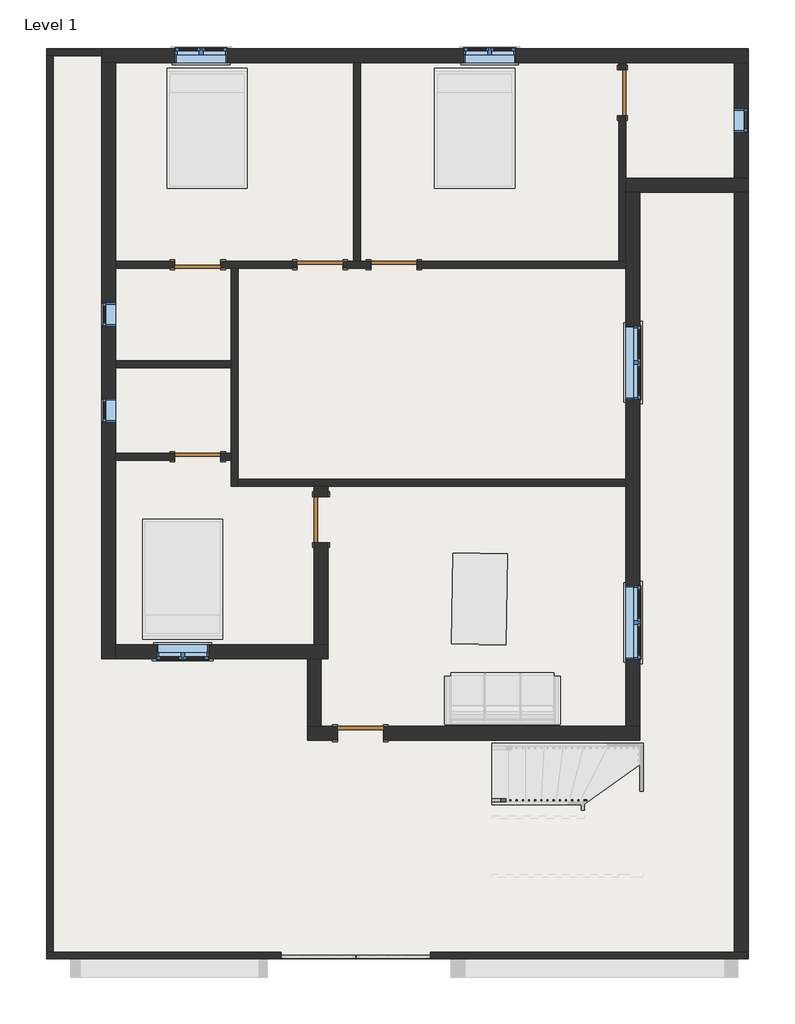
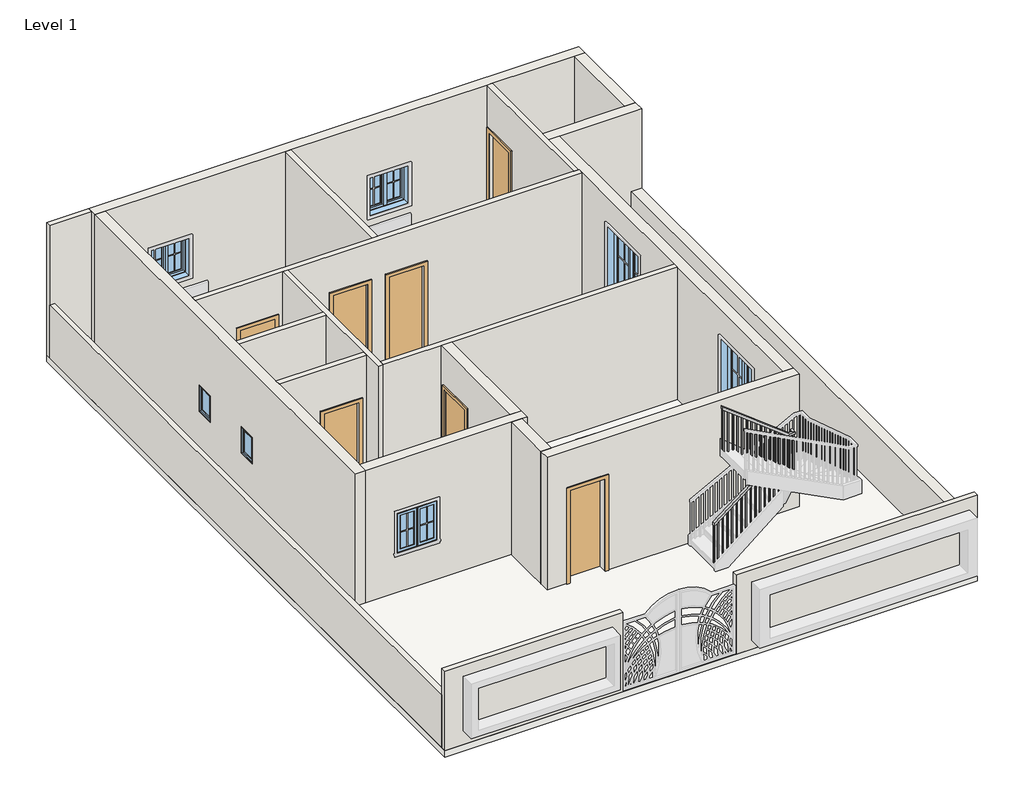
# One storey, part 1 of 2: 21 walls, 8 windows, 7 doors, 1 railing, 1 slab.
"""IFC4 building model written with IfcOpenShell, lengths in millimetres."""

from ifc_helpers import new_model, si_unit, frame, origin, origin_with_axes, place, context, project, spatial, polyline, outline, extrude, faceted_brep, transform, mapped, element, save
from components import door_f2b275c1, door_d8f5dbb5, door_214872d5, door_78caadf7, door_bb98abfd, window_aa618e30, window_339605e1, window_8377141f

model = new_model("IFC4")

# Units and contexts
model_context = context("Model", 3, world=origin())
ifc_project = project(units=[si_unit("LENGTHUNIT", "METRE", prefix="MILLI")], contexts=[model_context])

# Site, building, storey
site = spatial("IfcSite", under=ifc_project)
building = spatial("IfcBuilding", under=site)
storey = spatial("IfcBuildingStorey", under=building, Name="Level 1", Elevation=0.0)

# Doors
placement = place(None, origin())
door_shape = door_f2b275c1(model_context)
element("IfcDoor", 1, ObjectType="Single-Flush : 30\" x 80\"", at=placement, inside=storey, context=model_context, shape_type="MappedRepresentation", body=[
    mapped(door_shape, transform((2459.5084916, 7319.9935985, 0.0), x_axis=(0.0, 1.0, 0.0), y_axis=(-1.0, 0.0, 0.0), z_axis=(0.0, 0.0, 1.0))),
])
element("IfcDoor", 2, ObjectType="Single-Flush : 30\" x 80\"", at=placement, inside=storey, context=model_context, shape_type="MappedRepresentation", body=[
    mapped(door_shape, transform((-4550.8915084, 4481.5435985, 0.0), x_axis=(1.0, 0.0, 0.0), y_axis=(0.0, 1.0, 0.0), z_axis=(0.0, 0.0, 1.0))),
])
door_2_shape = door_d8f5dbb5(model_context)
element("IfcDoor", 3, ObjectType="Single-Flush : 30\" x 80\"", at=placement, inside=storey, context=model_context, shape_type="MappedRepresentation", body=[
    mapped(door_2_shape, transform((-4550.8915084, 1319.2435985, 0.0), x_axis=(1.0, 0.0, 0.0), y_axis=(0.0, 1.0, 0.0), z_axis=(0.0, 0.0, 1.0))),
])
door_3_shape = door_214872d5(model_context)
element("IfcDoor", 4, ObjectType="Single-Flush : 30\" x 84\"", at=placement, inside=storey, context=model_context, shape_type="MappedRepresentation", body=[
    mapped(door_3_shape, transform((-2531.5915084, 4481.5435985, 0.0), x_axis=(1.0, 0.0, 0.0), y_axis=(0.0, 1.0, 0.0), z_axis=(0.0, 0.0, 1.0))),
])
door_4_shape = door_78caadf7(model_context)
element("IfcDoor", 5, ObjectType="Single-Flush : 30\" x 84\"", at=placement, inside=storey, context=model_context, shape_type="MappedRepresentation", body=[
    mapped(door_4_shape, transform((-1312.3915084, 4481.5435985, 0.0), x_axis=(-1.0, 0.0, 0.0), y_axis=(0.0, -1.0, 0.0), z_axis=(0.0, 0.0, 1.0))),
])
door_5_shape = door_bb98abfd(model_context)
element("IfcDoor", 6, ObjectType="Single-Flush : 30\" x 84\"", at=placement, inside=storey, context=model_context, shape_type="MappedRepresentation", body=[
    mapped(door_5_shape, transform((-2512.5415084, 277.8435985, 0.0), x_axis=(0.0, 1.0, 0.0), y_axis=(-1.0, 0.0, 0.0), z_axis=(0.0, 0.0, 1.0))),
])
element("IfcDoor", 7, ObjectType="Single-Flush : 30\" x 84\"", at=placement, inside=storey, context=model_context, shape_type="MappedRepresentation", body=[
    mapped(door_5_shape, transform((-1864.8415084, -3246.4064015, 0.0), x_axis=(1.0, 0.0, 0.0), y_axis=(0.0, 1.0, 0.0), z_axis=(0.0, 0.0, 1.0))),
])

# Railing
element("IfcRailing", 8, ObjectType="Handrail - Rectangular", at=placement, inside=storey, context=model_context, shape_type="SolidModel", body=[
    faceted_brep([(306.9570026, -4325.9064015, 1083.7333333), (306.9570026, -4325.9064015, 1019.4000346), (306.9570026, -4376.7064015, 1019.4000346), (306.9570026, -4376.7064015, 1083.7333333), (1758.4886944, -4325.9064015, 2211.6191036), (1809.2886944, -4325.9064015, 2186.7590024), (1809.2886944, -4376.7064015, 2186.7590024), (1758.4886944, -4376.7064015, 2211.6191036), (1758.4886944, -4325.9064015, 2414.6281882), (1809.2886944, -4325.9064015, 2363.8281882), (1809.2886944, -4376.7064015, 2363.8281882), (1758.4886944, -4376.7064015, 2414.6281882), (1885.4886944, -4325.9064015, 2414.6281882), (1885.4886944, -4325.9064015, 2363.8281882), (1834.6886944, -4376.7064015, 2363.8281882), (1834.6886944, -4376.7064015, 2414.6281882), (1885.4886944, -4452.9064015, 2414.6281882), (1885.4886944, -4482.0277354, 2363.8281882), (1834.6886944, -4482.0277354, 2363.8281882), (1834.6886944, -4452.9064015, 2414.6281882), (1885.4886944, -4579.9064015, 2631.5051451), (1885.4886944, -4630.7064015, 2617.7256424), (1834.6886944, -4630.7064015, 2617.7256424), (1834.6886944, -4579.9064015, 2631.5051451), (1885.4886944, -4579.9064015, 2834.5142297), (1885.4886944, -4630.7064015, 2783.7142297), (1834.6886944, -4630.7064015, 2783.7142297), (1834.6886944, -4579.9064015, 2834.5142297), (1885.4886944, -4706.9064015, 2834.5142297), (1885.4886944, -4706.9064015, 2783.7142297), (1834.6886944, -4656.1064015, 2783.7142297), (1834.6886944, -4656.1064015, 2834.5142297), (1758.4886944, -4706.9064015, 2834.5142297), (1741.0720265, -4706.9064015, 2783.7142297), (1741.0720265, -4656.1064015, 2783.7142297), (1758.4886944, -4656.1064015, 2834.5142297), (306.9570026, -4706.9064015, 3962.4), (306.9570026, -4656.1064015, 3962.4), (306.9570026, -4656.1064015, 3898.0667013), (306.9570026, -4706.9064015, 3898.0667013)], [[[0, 1, 2, 3]], [[1, 0, 4, 5]], [[2, 1, 5, 6]], [[3, 2, 6, 7]], [[0, 3, 7, 4]], [[5, 4, 8, 9]], [[6, 5, 9, 10]], [[7, 6, 10, 11]], [[4, 7, 11, 8]], [[9, 8, 12, 13]], [[10, 9, 13, 14]], [[11, 10, 14, 15]], [[8, 11, 15, 12]], [[13, 12, 16, 17]], [[14, 13, 17, 18]], [[15, 14, 18, 19]], [[12, 15, 19, 16]], [[17, 16, 20, 21]], [[18, 17, 21, 22]], [[19, 18, 22, 23]], [[16, 19, 23, 20]], [[21, 20, 24, 25]], [[22, 21, 25, 26]], [[23, 22, 26, 27]], [[20, 23, 27, 24]], [[25, 24, 28, 29]], [[26, 25, 29, 30]], [[27, 26, 30, 31]], [[24, 27, 31, 28]], [[29, 28, 32, 33]], [[30, 29, 33, 34]], [[31, 30, 34, 35]], [[28, 31, 35, 32]], [[36, 37, 38, 39]], [[33, 32, 36, 39]], [[34, 33, 39, 38]], [[35, 34, 38, 37]], [[32, 35, 37, 36]]]),
    extrude(outline(polyline([(3868.0292361, 345.6136944), (3882.8316852, 326.5636944), (2878.6666667, 326.5636944), (2878.6666667, 345.6136944), (3868.0292361, 345.6136944)])), frame((0.0, -4691.0314015, 0.0), z_axis=(0.0, 1.0, 0.0), x_axis=(0.0, 0.0, 1.0)), (0.0, 0.0, 1.0), 19.05),
    extrude(outline(polyline([(3789.0828411, 447.2136944), (3803.8852902, 428.1636944), (2878.6666667, 428.1636944), (2878.6666667, 447.2136944), (3789.0828411, 447.2136944)])), frame((0.0, -4691.0314015, 0.0), z_axis=(0.0, 1.0, 0.0), x_axis=(0.0, 0.0, 1.0)), (0.0, 0.0, 1.0), 19.05),
    extrude(outline(polyline([(3710.1364462, 548.8136944), (3724.9388952, 529.7636944), (2878.6666667, 529.7636944), (2878.6666667, 548.8136944), (3710.1364462, 548.8136944)])), frame((0.0, -4691.0314015, 0.0), z_axis=(0.0, 1.0, 0.0), x_axis=(0.0, 0.0, 1.0)), (0.0, 0.0, 1.0), 19.05),
    extrude(outline(polyline([(3631.1900512, 650.4136944), (3645.9925003, 631.3636944), (2709.3333333, 631.3636944), (2709.3333333, 650.4136944), (3631.1900512, 650.4136944)])), frame((0.0, -4691.0314015, 0.0), z_axis=(0.0, 1.0, 0.0), x_axis=(0.0, 0.0, 1.0)), (0.0, 0.0, 1.0), 19.05),
    extrude(outline(polyline([(3552.2436562, 752.0136944), (3567.0461053, 732.9636944), (2709.3333333, 732.9636944), (2709.3333333, 752.0136944), (3552.2436562, 752.0136944)])), frame((0.0, -4691.0314015, 0.0), z_axis=(0.0, 1.0, 0.0), x_axis=(0.0, 0.0, 1.0)), (0.0, 0.0, 1.0), 19.05),
    extrude(outline(polyline([(3473.2972613, 853.6136944), (3488.0997103, 834.5636944), (2709.3333333, 834.5636944), (2709.3333333, 853.6136944), (3473.2972613, 853.6136944)])), frame((0.0, -4691.0314015, 0.0), z_axis=(0.0, 1.0, 0.0), x_axis=(0.0, 0.0, 1.0)), (0.0, 0.0, 1.0), 19.05),
    extrude(outline(polyline([(3394.3508663, 955.2136944), (3409.1533154, 936.1636944), (2540.0, 936.1636944), (2540.0, 955.2136944), (3394.3508663, 955.2136944)])), frame((0.0, -4691.0314015, 0.0), z_axis=(0.0, 1.0, 0.0), x_axis=(0.0, 0.0, 1.0)), (0.0, 0.0, 1.0), 19.05),
    extrude(outline(polyline([(3315.4044713, 1056.8136944), (3330.2069204, 1037.7636944), (2540.0, 1037.7636944), (2540.0, 1056.8136944), (3315.4044713, 1056.8136944)])), frame((0.0, -4691.0314015, 0.0), z_axis=(0.0, 1.0, 0.0), x_axis=(0.0, 0.0, 1.0)), (0.0, 0.0, 1.0), 19.05),
    extrude(outline(polyline([(3236.4580764, 1158.4136944), (3251.2605254, 1139.3636944), (2370.6666667, 1139.3636944), (2370.6666667, 1158.4136944), (3236.4580764, 1158.4136944)])), frame((0.0, -4691.0314015, 0.0), z_axis=(0.0, 1.0, 0.0), x_axis=(0.0, 0.0, 1.0)), (0.0, 0.0, 1.0), 19.05),
    extrude(outline(polyline([(3157.5116814, 1260.0136944), (3172.3141304, 1240.9636944), (2370.6666667, 1240.9636944), (2370.6666667, 1260.0136944), (3157.5116814, 1260.0136944)])), frame((0.0, -4691.0314015, 0.0), z_axis=(0.0, 1.0, 0.0), x_axis=(0.0, 0.0, 1.0)), (0.0, 0.0, 1.0), 19.05),
    extrude(outline(polyline([(3078.5652864, 1361.6136944), (3093.3677355, 1342.5636944), (2370.6666667, 1342.5636944), (2370.6666667, 1361.6136944), (3078.5652864, 1361.6136944)])), frame((0.0, -4691.0314015, 0.0), z_axis=(0.0, 1.0, 0.0), x_axis=(0.0, 0.0, 1.0)), (0.0, 0.0, 1.0), 19.05),
    extrude(outline(polyline([(2999.6188914, 1463.2136944), (3014.4213405, 1444.1636944), (2201.3333333, 1444.1636944), (2201.3333333, 1463.2136944), (2999.6188914, 1463.2136944)])), frame((0.0, -4691.0314015, 0.0), z_axis=(0.0, 1.0, 0.0), x_axis=(0.0, 0.0, 1.0)), (0.0, 0.0, 1.0), 19.05),
    extrude(outline(polyline([(2920.6724965, 1564.8136944), (2935.4749455, 1545.7636944), (2201.3333333, 1545.7636944), (2201.3333333, 1564.8136944), (2920.6724965, 1564.8136944)])), frame((0.0, -4691.0314015, 0.0), z_axis=(0.0, 1.0, 0.0), x_axis=(0.0, 0.0, 1.0)), (0.0, 0.0, 1.0), 19.05),
    extrude(outline(polyline([(2841.7261015, 1666.4136944), (2856.5285506, 1647.3636944), (2032.0, 1647.3636944), (2032.0, 1666.4136944), (2841.7261015, 1666.4136944)])), frame((0.0, -4691.0314015, 0.0), z_axis=(0.0, 1.0, 0.0), x_axis=(0.0, 0.0, 1.0)), (0.0, 0.0, 1.0), 19.05),
    extrude(outline(polyline([(2762.7797065, 1768.0136944), (2777.5821556, 1748.9636944), (2032.0, 1748.9636944), (2032.0, 1768.0136944), (2762.7797065, 1768.0136944)])), frame((0.0, -4691.0314015, 0.0), z_axis=(0.0, 1.0, 0.0), x_axis=(0.0, 0.0, 1.0)), (0.0, 0.0, 1.0), 19.05),
    extrude(outline(polyline([(1850.5636944, -4646.5814015), (1869.6136944, -4646.5814015), (1869.6136944, -4665.6314015), (1850.5636944, -4665.6314015), (1850.5636944, -4646.5814015)])), frame((0.0, 0.0, 1693.3333333), z_axis=(0.0, 0.0, 1.0), x_axis=(1.0, 0.0, 0.0)), (0.0, 0.0, 1.0), 1090.3808964),
    extrude(outline(polyline([(-4564.0314015, 2503.86524), (-4544.9814015, 2471.3336964), (-4544.9814015, 1524.0), (-4564.0314015, 1524.0), (-4564.0314015, 2503.86524)])), frame((1850.5636944, 0.0, 0.0), z_axis=(1.0, 0.0, 0.0), x_axis=(0.0, 1.0, 0.0)), (0.0, 0.0, 1.0), 19.05),
    extrude(outline(polyline([(-4462.4314015, 2330.3636744), (-4443.3814015, 2297.8321309), (-4443.3814015, 1354.6666667), (-4462.4314015, 1354.6666667), (-4462.4314015, 2330.3636744)])), frame((1850.5636944, 0.0, 0.0), z_axis=(1.0, 0.0, 0.0), x_axis=(0.0, 1.0, 0.0)), (0.0, 0.0, 1.0), 19.05),
    extrude(outline(polyline([(1821.4320026, -4360.8314015), (1821.4320026, -4341.7814015), (1840.4820026, -4341.7814015), (1840.4820026, -4360.8314015), (1821.4320026, -4360.8314015)])), frame((0.0, 0.0, 1185.3333333), z_axis=(0.0, 0.0, 1.0), x_axis=(1.0, 0.0, 0.0)), (0.0, 0.0, 1.0), 1178.4948549),
    extrude(outline(polyline([(2132.0507888, 1738.8820026), (2117.2483397, 1719.8320026), (1016.0, 1719.8320026), (1016.0, 1738.8820026), (2132.0507888, 1738.8820026)])), frame((0.0, -4360.8314015, 0.0), z_axis=(0.0, 1.0, 0.0), x_axis=(0.0, 0.0, 1.0)), (0.0, 0.0, 1.0), 19.05),
    extrude(outline(polyline([(2053.1043938, 1637.2820026), (2038.3019447, 1618.2320026), (1016.0, 1618.2320026), (1016.0, 1637.2820026), (2053.1043938, 1637.2820026)])), frame((0.0, -4360.8314015, 0.0), z_axis=(0.0, 1.0, 0.0), x_axis=(0.0, 0.0, 1.0)), (0.0, 0.0, 1.0), 19.05),
    extrude(outline(polyline([(1974.1579988, 1535.6820026), (1959.3555498, 1516.6320026), (846.6666667, 1516.6320026), (846.6666667, 1535.6820026), (1974.1579988, 1535.6820026)])), frame((0.0, -4360.8314015, 0.0), z_axis=(0.0, 1.0, 0.0), x_axis=(0.0, 0.0, 1.0)), (0.0, 0.0, 1.0), 19.05),
    extrude(outline(polyline([(1895.2116039, 1434.0820026), (1880.4091548, 1415.0320026), (846.6666667, 1415.0320026), (846.6666667, 1434.0820026), (1895.2116039, 1434.0820026)])), frame((0.0, -4360.8314015, 0.0), z_axis=(0.0, 1.0, 0.0), x_axis=(0.0, 0.0, 1.0)), (0.0, 0.0, 1.0), 19.05),
    extrude(outline(polyline([(1816.2652089, 1332.4820026), (1801.4627598, 1313.4320026), (677.3333333, 1313.4320026), (677.3333333, 1332.4820026), (1816.2652089, 1332.4820026)])), frame((0.0, -4360.8314015, 0.0), z_axis=(0.0, 1.0, 0.0), x_axis=(0.0, 0.0, 1.0)), (0.0, 0.0, 1.0), 19.05),
    extrude(outline(polyline([(1737.3188139, 1230.8820026), (1722.5163649, 1211.8320026), (677.3333333, 1211.8320026), (677.3333333, 1230.8820026), (1737.3188139, 1230.8820026)])), frame((0.0, -4360.8314015, 0.0), z_axis=(0.0, 1.0, 0.0), x_axis=(0.0, 0.0, 1.0)), (0.0, 0.0, 1.0), 19.05),
    extrude(outline(polyline([(1658.3724189, 1129.2820026), (1643.5699699, 1110.2320026), (508.0, 1110.2320026), (508.0, 1129.2820026), (1658.3724189, 1129.2820026)])), frame((0.0, -4360.8314015, 0.0), z_axis=(0.0, 1.0, 0.0), x_axis=(0.0, 0.0, 1.0)), (0.0, 0.0, 1.0), 19.05),
    extrude(outline(polyline([(1579.426024, 1027.6820026), (1564.6235749, 1008.6320026), (508.0, 1008.6320026), (508.0, 1027.6820026), (1579.426024, 1027.6820026)])), frame((0.0, -4360.8314015, 0.0), z_axis=(0.0, 1.0, 0.0), x_axis=(0.0, 0.0, 1.0)), (0.0, 0.0, 1.0), 19.05),
    extrude(outline(polyline([(1500.479629, 926.0820026), (1485.6771799, 907.0320026), (508.0, 907.0320026), (508.0, 926.0820026), (1500.479629, 926.0820026)])), frame((0.0, -4360.8314015, 0.0), z_axis=(0.0, 1.0, 0.0), x_axis=(0.0, 0.0, 1.0)), (0.0, 0.0, 1.0), 19.05),
    extrude(outline(polyline([(1421.533234, 824.4820026), (1406.730785, 805.4320026), (338.6666667, 805.4320026), (338.6666667, 824.4820026), (1421.533234, 824.4820026)])), frame((0.0, -4360.8314015, 0.0), z_axis=(0.0, 1.0, 0.0), x_axis=(0.0, 0.0, 1.0)), (0.0, 0.0, 1.0), 19.05),
    extrude(outline(polyline([(1342.5868391, 722.8820026), (1327.78439, 703.8320026), (338.6666667, 703.8320026), (338.6666667, 722.8820026), (1342.5868391, 722.8820026)])), frame((0.0, -4360.8314015, 0.0), z_axis=(0.0, 1.0, 0.0), x_axis=(0.0, 0.0, 1.0)), (0.0, 0.0, 1.0), 19.05),
    extrude(outline(polyline([(1263.6404441, 621.2820026), (1248.837995, 602.2320026), (338.6666667, 602.2320026), (338.6666667, 621.2820026), (1263.6404441, 621.2820026)])), frame((0.0, -4360.8314015, 0.0), z_axis=(0.0, 1.0, 0.0), x_axis=(0.0, 0.0, 1.0)), (0.0, 0.0, 1.0), 19.05),
    extrude(outline(polyline([(1184.6940491, 519.6820026), (1169.8916001, 500.6320026), (169.3333333, 500.6320026), (169.3333333, 519.6820026), (1184.6940491, 519.6820026)])), frame((0.0, -4360.8314015, 0.0), z_axis=(0.0, 1.0, 0.0), x_axis=(0.0, 0.0, 1.0)), (0.0, 0.0, 1.0), 19.05),
    extrude(outline(polyline([(1105.7476541, 418.0820026), (1090.9452051, 399.0320026), (169.3333333, 399.0320026), (169.3333333, 418.0820026), (1105.7476541, 418.0820026)])), frame((0.0, -4360.8314015, 0.0), z_axis=(0.0, 1.0, 0.0), x_axis=(0.0, 0.0, 1.0)), (0.0, 0.0, 1.0), 19.05),
    extrude(outline(polyline([(1850.5636944, -4671.9814015), (1869.6136944, -4671.9814015), (1869.6136944, -4691.0314015), (1850.5636944, -4691.0314015), (1850.5636944, -4671.9814015)])), frame((0.0, 0.0, 1862.6666667), z_axis=(0.0, 0.0, 1.0), x_axis=(1.0, 0.0, 0.0)), (0.0, 0.0, 1.0), 921.0475631),
    extrude(outline(polyline([(1850.5636944, -4360.8314015), (1850.5636944, -4341.7814015), (1869.6136944, -4341.7814015), (1869.6136944, -4360.8314015), (1850.5636944, -4360.8314015)])), frame((0.0, 0.0, 1185.3333333), z_axis=(0.0, 0.0, 1.0), x_axis=(1.0, 0.0, 0.0)), (0.0, 0.0, 1.0), 1178.4948549),
    extrude(outline(polyline([(3883.2642523, 326.0070026), (3898.0667013, 306.9570026), (2878.6666667, 306.9570026), (2878.6666667, 326.0070026), (3883.2642523, 326.0070026)])), frame((0.0, -4691.0314015, 0.0), z_axis=(0.0, 1.0, 0.0), x_axis=(0.0, 0.0, 1.0)), (0.0, 0.0, 1.0), 19.05),
    extrude(outline(polyline([(1034.2024837, 326.0070026), (1019.4000346, 306.9570026), (169.3333333, 306.9570026), (169.3333333, 326.0070026), (1034.2024837, 326.0070026)])), frame((0.0, -4360.8314015, 0.0), z_axis=(0.0, 1.0, 0.0), x_axis=(0.0, 0.0, 1.0)), (0.0, 0.0, 1.0), 19.05),
])

# Slab
element("IfcSlab", 9, ObjectType="Generic - 12\"", at=placement, inside=storey, context=model_context, shape_type="SweptSolid", body=[
    extrude(outline(polyline([(4535.9584916, 8043.8940003), (4535.9584916, -6967.5064015), (-7046.4415084, -6967.5064015), (-7046.4415084, 8043.8940003), (4535.9584916, 8043.8940003)])), frame((0.0, 0.0, -152.4), z_axis=(0.0, 0.0, 1.0), x_axis=(1.0, 0.0, 0.0)), (0.0, 0.0, 1.0), 152.4),
])

# Walls
element("IfcWall", 10, ObjectType="WALL4.5\"", at=placement, inside=storey, context=model_context, shape_type="SweptSolid", body=[
    extrude(outline(polyline([(-1979.1415084, 4538.6935985), (-1979.1415084, 7815.2935985), (-1864.8415084, 7815.2935985), (-1864.8415084, 4538.6935985), (-1979.1415084, 4538.6935985)])), origin_with_axes(), (0.0, 0.0, 1.0), 3048.0),
])
element("IfcWall", 11, ObjectType="WALL4.5\"", at=placement, inside=storey, context=model_context, shape_type="Brep", body=[
    faceted_brep([(-2150.5915084, 4424.3935985, 0.0), (-1693.3915084, 4424.3935985, 0.0), (-1693.3915084, 4424.3935985, 2133.6), (-931.3915084, 4424.3935985, 2133.6), (-931.3915084, 4424.3935985, 0.0), (2516.6584916, 4424.3935985, 0.0), (2516.6584916, 4424.3935985, 3048.0), (-3884.1415084, 4424.3935985, 3048.0), (-3998.4415084, 4424.3935985, 3048.0), (-5903.4415084, 4424.3935985, 3048.0), (-5903.4415084, 4424.3935985, 0.0), (-4931.8915084, 4424.3935985, 0.0), (-4931.8915084, 4424.3935985, 2032.0), (-4169.8915084, 4424.3935985, 2032.0), (-4169.8915084, 4424.3935985, 0.0), (-3998.4415084, 4424.3935985, 0.0), (-3884.1415084, 4424.3935985, 0.0), (-2912.5915084, 4424.3935985, 0.0), (-2912.5915084, 4424.3935985, 2133.6), (-2150.5915084, 4424.3935985, 2133.6), (-1693.3915084, 4538.6935985, 2133.6), (-1693.3915084, 4538.6935985, 0.0), (-1864.8415084, 4538.6935985, 0.0), (-1979.1415084, 4538.6935985, 0.0), (-2150.5915084, 4538.6935985, 0.0), (-2150.5915084, 4538.6935985, 2133.6), (-2912.5915084, 4538.6935985, 2133.6), (-2912.5915084, 4538.6935985, 0.0), (-4169.8915084, 4538.6935985, 0.0), (-4169.8915084, 4538.6935985, 2032.0), (-4931.8915084, 4538.6935985, 2032.0), (-4931.8915084, 4538.6935985, 0.0), (-5903.4415084, 4538.6935985, 0.0), (-5903.4415084, 4538.6935985, 3048.0), (-1979.1415084, 4538.6935985, 3048.0), (-1864.8415084, 4538.6935985, 3048.0), (2402.3584916, 4538.6935985, 3048.0), (2516.6584916, 4538.6935985, 3048.0), (2516.6584916, 4538.6935985, 0.0), (2402.3584916, 4538.6935985, 0.0), (-931.3915084, 4538.6935985, 0.0), (-931.3915084, 4538.6935985, 2133.6)], [[[0, 1, 2, 3, 4, 5, 6, 7, 8, 9, 10, 11, 12, 13, 14, 15, 16, 17, 18, 19]], [[20, 21, 22, 23, 24, 25, 26, 27, 28, 29, 30, 31, 32, 33, 34, 35, 36, 37, 38, 39, 40, 41]], [[11, 10, 32, 31]], [[17, 16, 15, 14, 28, 27]], [[40, 39, 38, 5, 4]], [[24, 23, 22, 21, 1, 0]], [[10, 9, 33, 32]], [[6, 5, 38, 37]], [[29, 28, 14, 13]], [[30, 29, 13, 12]], [[31, 30, 12, 11]], [[25, 24, 0, 19]], [[26, 25, 19, 18]], [[27, 26, 18, 17]], [[2, 1, 21, 20]], [[3, 2, 20, 41]], [[4, 3, 41, 40]], [[9, 8, 7, 6, 37, 36, 35, 34, 33]]]),
])
element("IfcWall", 12, ObjectType="WALL4.5\"", at=placement, inside=storey, context=model_context, shape_type="Brep", body=[
    faceted_brep([(2516.6584916, 7700.9935985, 2032.0), (2516.6584916, 7700.9935985, 0.0), (2516.6584916, 7815.2935985, 0.0), (2516.6584916, 7815.2935985, 3048.0), (2516.6584916, 5910.2935985, 3048.0), (2516.6584916, 5681.6935985, 3048.0), (2516.6584916, 4538.6935985, 3048.0), (2516.6584916, 4538.6935985, 0.0), (2516.6584916, 5681.6935985, 0.0), (2516.6584916, 5910.2935985, 0.0), (2516.6584916, 6938.9935985, 0.0), (2516.6584916, 6938.9935985, 2032.0), (2402.3584916, 7815.2935985, 0.0), (2402.3584916, 7700.9935985, 0.0), (2402.3584916, 7700.9935985, 2032.0), (2402.3584916, 6938.9935985, 2032.0), (2402.3584916, 6938.9935985, 0.0), (2402.3584916, 4538.6935985, 0.0), (2402.3584916, 4538.6935985, 3048.0), (2402.3584916, 7815.2935985, 3048.0)], [[[0, 1, 2, 3, 4, 5, 6, 7, 8, 9, 10, 11]], [[12, 13, 14, 15, 16, 17, 18, 19]], [[2, 1, 13, 12]], [[10, 9, 8, 7, 17, 16]], [[7, 6, 18, 17]], [[3, 2, 12, 19]], [[14, 13, 1, 0]], [[15, 14, 0, 11]], [[16, 15, 11, 10]], [[6, 5, 4, 3, 19, 18]]]),
])
element("IfcWall", 13, ObjectType="WALL4.5\"", at=placement, inside=storey, context=model_context, shape_type="Brep", body=[
    faceted_brep([(-3998.4415084, 4424.3935985, 0.0), (-3998.4415084, 2900.3935985, 0.0), (-3998.4415084, 2786.0935985, 0.0), (-3998.4415084, 1376.3935985, 0.0), (-3998.4415084, 1262.0935985, 0.0), (-3998.4415084, 830.2935985, 0.0), (-3998.4415084, 830.2935985, 3048.0), (-3998.4415084, 1262.0935985, 3048.0), (-3998.4415084, 1376.3935985, 3048.0), (-3998.4415084, 2786.0935985, 3048.0), (-3998.4415084, 2900.3935985, 3048.0), (-3998.4415084, 4424.3935985, 3048.0), (-3884.1415084, 4424.3935985, 0.0), (-3884.1415084, 4424.3935985, 3048.0), (-3884.1415084, 944.5935985, 3048.0), (-3884.1415084, 830.2935985, 3048.0), (-3884.1415084, 830.2935985, 0.0), (-3884.1415084, 944.5935985, 0.0)], [[[0, 1, 2, 3, 4, 5, 6, 7, 8, 9, 10, 11]], [[12, 13, 14, 15, 16, 17]], [[5, 4, 3, 2, 1, 0, 12, 17, 16]], [[0, 11, 13, 12]], [[6, 5, 16, 15]], [[11, 10, 9, 8, 7, 6, 15, 14, 13]]]),
])
element("IfcWall", 14, ObjectType="WALL4.5\"", at=placement, inside=storey, context=model_context, shape_type="Brep", body=[
    faceted_brep([(-3884.1415084, 830.2935985, 0.0), (-2626.8415084, 830.2935985, 0.0), (-2398.2415084, 830.2935985, 0.0), (2516.6584916, 830.2935985, 0.0), (2516.6584916, 830.2935985, 3048.0), (-2398.2415084, 830.2935985, 3048.0), (-2626.8415084, 830.2935985, 3048.0), (-3884.1415084, 830.2935985, 3048.0), (-3884.1415084, 944.5935985, 0.0), (-3884.1415084, 944.5935985, 3048.0), (2516.6584916, 944.5935985, 3048.0), (2516.6584916, 944.5935985, 0.0)], [[[0, 1, 2, 3, 4, 5, 6, 7]], [[8, 9, 10, 11]], [[3, 2, 1, 0, 8, 11]], [[0, 7, 9, 8]], [[4, 3, 11, 10]], [[7, 6, 5, 4, 10, 9]]]),
])
element("IfcWall", 15, ObjectType="WALL4.5\"", at=placement, inside=storey, context=model_context, shape_type="SweptSolid", body=[
    extrude(outline(polyline([(-3998.4415084, 2786.0935985), (-5903.4415084, 2786.0935985), (-5903.4415084, 2900.3935985), (-3998.4415084, 2900.3935985), (-3998.4415084, 2786.0935985)])), origin_with_axes(), (0.0, 0.0, 1.0), 3048.0),
])
element("IfcWall", 16, ObjectType="WALL4.5\"", at=placement, inside=storey, context=model_context, shape_type="SweptSolid", body=[
    extrude(outline(polyline([(2032.0, -4169.8915084), (0.0, -4169.8915084), (0.0, -3998.4415084), (3048.0, -3998.4415084), (3048.0, -5903.4415084), (0.0, -5903.4415084), (0.0, -4931.8915084), (2032.0, -4931.8915084), (2032.0, -4169.8915084)])), frame((0.0, 1262.0935985, 0.0), z_axis=(0.0, 1.0, 0.0), x_axis=(0.0, 0.0, 1.0)), (0.0, 0.0, 1.0), 114.3),
])
element("IfcWall", 17, ObjectType="WALL4.5\"", at=placement, inside=storey, context=model_context, shape_type="Brep", body=[
    faceted_brep([(-6132.0415084, 8043.8940003, 0.0), (-7046.4415084, 8043.8940003, 0.0), (-7046.4415084, 8043.8940003, 3048.0), (-6132.0415084, 8043.8940003, 3048.0), (-6132.0415084, 7929.5940003, 0.0), (-6132.0415084, 7929.5940003, 3048.0), (-7046.4415084, 7929.5940003, 3048.0), (-7046.4415084, 7929.5940003, 1219.2), (-7046.4415084, 7929.5940003, 0.0), (-6932.1415084, 7929.5940003, 0.0)], [[[0, 1, 2, 3]], [[4, 5, 6, 7, 8, 9]], [[1, 0, 4, 9, 8]], [[3, 2, 6, 5]], [[0, 3, 5, 4]], [[2, 1, 8, 7, 6]]]),
])
element("IfcWall", 18, ObjectType="WALL4.5\"", at=placement, inside=storey, context=model_context, shape_type="Brep", body=[
    faceted_brep([(-7046.4415084, -6967.5064015, 0.0), (-3179.2915084, -6967.5064015, 0.0), (-3179.2915084, -6967.5064015, 1828.8), (-7046.4415084, -6967.5064015, 1828.8), (-7046.4415084, -6853.2064015, 0.0), (-7046.4415084, -6853.2064015, 1219.2), (-7046.4415084, -6853.2064015, 1828.8), (-3179.2915084, -6853.2064015, 1828.8), (-3179.2915084, -6853.2064015, 0.0), (-6932.1415084, -6853.2064015, 0.0)], [[[0, 1, 2, 3]], [[4, 5, 6, 7, 8, 9]], [[1, 0, 4, 9, 8]], [[2, 1, 8, 7]], [[3, 2, 7, 6]], [[0, 3, 6, 5, 4]]]),
])
element("IfcWall", 19, ObjectType="WALL4.5\"", at=placement, inside=storey, context=model_context, shape_type="SweptSolid", body=[
    extrude(outline(polyline([(-7046.4415084, -6853.2064015), (-7046.4415084, 7929.5940003), (-6932.1415084, 7929.5940003), (-6932.1415084, -6853.2064015), (-7046.4415084, -6853.2064015)])), origin_with_axes(), (0.0, 0.0, 1.0), 1219.2),
])
element("IfcWall", 20, ObjectType="WALL4.5\"", at=placement, inside=storey, context=model_context, shape_type="Brep", body=[
    faceted_brep([(-709.1415084, -6967.5064015, 0.0), (4535.9584916, -6967.5064015, 0.0), (4535.9584916, -6967.5064015, 1828.8), (-709.1415084, -6967.5064015, 1828.8), (-709.1415084, -6853.2064015, 0.0), (-709.1415084, -6853.2064015, 1828.8), (4535.9584916, -6853.2064015, 1828.8), (4535.9584916, -6853.2064015, 1219.2), (4535.9584916, -6853.2064015, 0.0), (4307.3584916, -6853.2064015, 0.0)], [[[0, 1, 2, 3]], [[4, 5, 6, 7, 8, 9]], [[1, 0, 4, 9, 8]], [[3, 2, 6, 5]], [[0, 3, 5, 4]], [[2, 1, 8, 7, 6]]]),
])
element("IfcWall", 21, ObjectType="WALL9\"", at=placement, inside=storey, context=model_context, shape_type="Brep", body=[
    faceted_brep([(-6132.0415084, 7815.2935985, 0.0), (-5903.4415084, 7815.2935985, 0.0), (-1979.1415084, 7815.2935985, 0.0), (-1864.8415084, 7815.2935985, 0.0), (2402.3584916, 7815.2935985, 0.0), (2516.6584916, 7815.2935985, 0.0), (4307.3584916, 7815.2935985, 0.0), (4535.9584916, 7815.2935985, 0.0), (4535.9584916, 7815.2935985, 3048.0), (4307.3584916, 7815.2935985, 3048.0), (2516.6584916, 7815.2935985, 3048.0), (2402.3584916, 7815.2935985, 3048.0), (-1864.8415084, 7815.2935985, 3048.0), (-1979.1415084, 7815.2935985, 3048.0), (-5903.4415084, 7815.2935985, 3048.0), (-6132.0415084, 7815.2935985, 3048.0), (-4061.9415084, 7815.2935985, 1828.8), (-4061.9415084, 7815.2935985, 914.4), (-4925.5415084, 7815.2935985, 914.4), (-4925.5415084, 7815.2935985, 1828.8), (700.5584916, 7815.2935985, 1828.8), (700.5584916, 7815.2935985, 914.4), (-163.0415084, 7815.2935985, 914.4), (-163.0415084, 7815.2935985, 1828.8), (-6132.0415084, 8043.8935985, 0.0), (-6132.0415084, 8043.8935985, 3048.0), (4535.9584916, 8043.8935985, 3048.0), (4535.9584916, 8043.8935985, 0.0), (-4061.9415084, 8043.8935985, 1828.8), (-4925.5415084, 8043.8935985, 1828.8), (-4925.5415084, 8043.8935985, 914.4), (-4061.9415084, 8043.8935985, 914.4), (700.5584916, 8043.8935985, 1828.8), (-163.0415084, 8043.8935985, 1828.8), (-163.0415084, 8043.8935985, 914.4), (700.5584916, 8043.8935985, 914.4), (-6132.0415084, 7929.5940003, 0.0), (-6132.0415084, 7929.5940003, 3048.0)], [[[0, 1, 2, 3, 4, 5, 6, 7, 8, 9, 10, 11, 12, 13, 14, 15], [16, 17, 18, 19], [20, 21, 22, 23]], [[24, 25, 26, 27], [28, 29, 30, 31], [32, 33, 34, 35]], [[7, 6, 5, 4, 3, 2, 1, 0, 36, 24, 27]], [[0, 15, 37, 25, 24, 36]], [[8, 7, 27, 26]], [[17, 16, 28, 31]], [[18, 17, 31, 30]], [[19, 18, 30, 29]], [[16, 19, 29, 28]], [[21, 20, 32, 35]], [[22, 21, 35, 34]], [[23, 22, 34, 33]], [[20, 23, 33, 32]], [[15, 14, 13, 12, 11, 10, 9, 8, 26, 25, 37]]]),
])
element("IfcWall", 22, ObjectType="WALL9\"", at=placement, inside=storey, context=model_context, shape_type="Brep", body=[
    faceted_brep([(-6132.0415084, 7815.2935985, 0.0), (-6132.0415084, -2014.5064015, 0.0), (-6132.0415084, -2014.5064015, 3048.0), (-6132.0415084, 7815.2935985, 3048.0), (-6132.0415084, 3865.5935985, 1524.0), (-6132.0415084, 3459.1935985, 1524.0), (-6132.0415084, 3459.1935985, 914.4), (-6132.0415084, 3865.5935985, 914.4), (-6132.0415084, 2284.4435985, 1524.0), (-6132.0415084, 1878.0435985, 1524.0), (-6132.0415084, 1878.0435985, 914.4), (-6132.0415084, 2284.4435985, 914.4), (-5903.4415084, 7815.2935985, 0.0), (-5903.4415084, 7815.2935985, 3048.0), (-5903.4415084, 4538.6935985, 3048.0), (-5903.4415084, 4424.3935985, 3048.0), (-5903.4415084, 2900.3935985, 3048.0), (-5903.4415084, 2786.0935985, 3048.0), (-5903.4415084, 1376.3935985, 3048.0), (-5903.4415084, 1262.0935985, 3048.0), (-5903.4415084, -1785.9064015, 3048.0), (-5903.4415084, -2014.5064015, 3048.0), (-5903.4415084, -2014.5064015, 0.0), (-5903.4415084, -1785.9064015, 0.0), (-5903.4415084, 1262.0935985, 0.0), (-5903.4415084, 1376.3935985, 0.0), (-5903.4415084, 2786.0935985, 0.0), (-5903.4415084, 2900.3935985, 0.0), (-5903.4415084, 4424.3935985, 0.0), (-5903.4415084, 4538.6935985, 0.0), (-5903.4415084, 3865.5935985, 1524.0), (-5903.4415084, 3865.5935985, 914.4), (-5903.4415084, 3459.1935985, 914.4), (-5903.4415084, 3459.1935985, 1524.0), (-5903.4415084, 2284.4435985, 1524.0), (-5903.4415084, 2284.4435985, 914.4), (-5903.4415084, 1878.0435985, 914.4), (-5903.4415084, 1878.0435985, 1524.0)], [[[0, 1, 2, 3], [4, 5, 6, 7], [8, 9, 10, 11]], [[12, 13, 14, 15, 16, 17, 18, 19, 20, 21, 22, 23, 24, 25, 26, 27, 28, 29], [30, 31, 32, 33], [34, 35, 36, 37]], [[1, 0, 12, 29, 28, 27, 26, 25, 24, 23, 22]], [[0, 3, 13, 12]], [[2, 1, 22, 21]], [[31, 30, 4, 7]], [[32, 31, 7, 6]], [[33, 32, 6, 5]], [[30, 33, 5, 4]], [[35, 34, 8, 11]], [[36, 35, 11, 10]], [[37, 36, 10, 9]], [[34, 37, 9, 8]], [[3, 2, 21, 20, 19, 18, 17, 16, 15, 14, 13]]]),
])
element("IfcWall", 23, ObjectType="WALL9\"", at=placement, inside=storey, context=model_context, shape_type="Brep", body=[
    faceted_brep([(-5903.4415084, -2014.5064015, 0.0), (-2741.1415084, -2014.5064015, 0.0), (-2512.5415084, -2014.5064015, 0.0), (-2398.2415084, -2014.5064015, 0.0), (-2398.2415084, -2014.5064015, 3048.0), (-2512.5415084, -2014.5064015, 3048.0), (-2741.1415084, -2014.5064015, 3048.0), (-5903.4415084, -2014.5064015, 3048.0), (-5230.3415084, -2014.5064015, 1828.8), (-4366.7415084, -2014.5064015, 1828.8), (-4366.7415084, -2014.5064015, 914.4), (-5230.3415084, -2014.5064015, 914.4), (-5903.4415084, -1785.9064015, 0.0), (-5903.4415084, -1785.9064015, 3048.0), (-2626.8415084, -1785.9064015, 3048.0), (-2398.2415084, -1785.9064015, 3048.0), (-2398.2415084, -1785.9064015, 0.0), (-2626.8415084, -1785.9064015, 0.0), (-5230.3415084, -1785.9064015, 1828.8), (-5230.3415084, -1785.9064015, 914.4), (-4366.7415084, -1785.9064015, 914.4), (-4366.7415084, -1785.9064015, 1828.8)], [[[0, 1, 2, 3, 4, 5, 6, 7], [8, 9, 10, 11]], [[12, 13, 14, 15, 16, 17], [18, 19, 20, 21]], [[3, 2, 1, 0, 12, 17, 16]], [[0, 7, 13, 12]], [[4, 3, 16, 15]], [[19, 18, 8, 11]], [[20, 19, 11, 10]], [[21, 20, 10, 9]], [[18, 21, 9, 8]], [[7, 6, 5, 4, 15, 14, 13]]]),
])
element("IfcWall", 24, ObjectType="WALL9\"", at=placement, inside=storey, context=model_context, shape_type="SweptSolid", body=[
    extrude(outline(polyline([(830.2935985, 0.0), (658.8435985, 0.0), (658.8435985, 2133.6), (-103.1564015, 2133.6), (-103.1564015, 0.0), (-1785.9064015, 0.0), (-1785.9064015, 3048.0), (830.2935985, 3048.0), (830.2935985, 0.0)])), frame((-2626.8415084, 0.0, 0.0), z_axis=(1.0, 0.0, 0.0), x_axis=(0.0, 1.0, 0.0)), (0.0, 0.0, 1.0), 228.6),
])
element("IfcWall", 25, ObjectType="WALL9\"", at=placement, inside=storey, context=model_context, shape_type="Brep", body=[
    faceted_brep([(2745.2584916, -3132.1064015, 0.0), (2516.6584916, -3132.1064015, 0.0), (-1483.8415084, -3132.1064015, 0.0), (-1483.8415084, -3132.1064015, 2133.6), (-2245.8415084, -3132.1064015, 2133.6), (-2245.8415084, -3132.1064015, 0.0), (-2512.5415084, -3132.1064015, 0.0), (-2741.1415084, -3132.1064015, 0.0), (-2741.1415084, -3132.1064015, 3048.0), (-2512.5415084, -3132.1064015, 3048.0), (2516.6584916, -3132.1064015, 3048.0), (2745.2584916, -3132.1064015, 3048.0), (-1483.8415084, -3360.7064015, 2133.6), (-1483.8415084, -3360.7064015, 0.0), (2745.2584916, -3360.7064015, 0.0), (2745.2584916, -3360.7064015, 3048.0), (-2741.1415084, -3360.7064015, 3048.0), (-2741.1415084, -3360.7064015, 0.0), (-2245.8415084, -3360.7064015, 0.0), (-2245.8415084, -3360.7064015, 2133.6)], [[[0, 1, 2, 3, 4, 5, 6, 7, 8, 9, 10, 11]], [[12, 13, 14, 15, 16, 17, 18, 19]], [[18, 17, 7, 6, 5]], [[14, 13, 2, 1, 0]], [[8, 7, 17, 16]], [[0, 11, 15, 14]], [[3, 2, 13, 12]], [[4, 3, 12, 19]], [[5, 4, 19, 18]], [[11, 10, 9, 8, 16, 15]]]),
])
element("IfcWall", 26, ObjectType="WALL9\"", at=placement, inside=storey, context=model_context, shape_type="SweptSolid", body=[
    extrude(outline(polyline([(-2512.5415084, -2014.5064015), (-2512.5415084, -3132.1064015), (-2741.1415084, -3132.1064015), (-2741.1415084, -2014.5064015), (-2512.5415084, -2014.5064015)])), origin_with_axes(), (0.0, 0.0, 1.0), 3048.0),
])
element("IfcWall", 27, ObjectType="WALL9\"", at=placement, inside=storey, context=model_context, shape_type="Brep", body=[
    faceted_brep([(4535.9584916, 5910.2935985, 3048.0), (4535.9584916, 5910.2935985, 0.0), (4307.3584916, 5910.2935985, 0.0), (2516.6584916, 5910.2935985, 0.0), (2516.6584916, 5910.2935985, 3048.0), (4307.3584916, 5910.2935985, 3048.0), (4535.9584916, 5681.6935985, 0.0), (4535.9584916, 5681.6935985, 1219.2), (4535.9584916, 5681.6935985, 3048.0), (2745.2584916, 5681.6935985, 3048.0), (2516.6584916, 5681.6935985, 3048.0), (2516.6584916, 5681.6935985, 0.0), (2745.2584916, 5681.6935985, 0.0), (4307.3584916, 5681.6935985, 0.0)], [[[0, 1, 2, 3, 4, 5]], [[6, 7, 8, 9, 10, 11, 12, 13]], [[3, 2, 1, 6, 13, 12, 11]], [[4, 3, 11, 10]], [[0, 8, 7, 6, 1]], [[0, 5, 4, 10, 9, 8]]]),
])
element("IfcWall", 28, ObjectType="WALL9\"", at=placement, inside=storey, context=model_context, shape_type="Brep", body=[
    faceted_brep([(2516.6584916, 5681.6935985, 0.0), (2516.6584916, 944.5935985, 0.0), (2516.6584916, 830.2935985, 0.0), (2516.6584916, -3132.1064015, 0.0), (2516.6584916, -3132.1064015, 3048.0), (2516.6584916, 830.2935985, 3048.0), (2516.6584916, 944.5935985, 3048.0), (2516.6584916, 5681.6935985, 3048.0), (2516.6584916, -2027.2064015, 2438.4), (2516.6584916, -2027.2064015, 914.4), (2516.6584916, -808.0064015, 914.4), (2516.6584916, -808.0064015, 2438.4), (2516.6584916, 2259.0435985, 2438.4), (2516.6584916, 2259.0435985, 914.4), (2516.6584916, 3478.2435985, 914.4), (2516.6584916, 3478.2435985, 2438.4), (2745.2584916, 5681.6935985, 0.0), (2745.2584916, 5681.6935985, 3048.0), (2745.2584916, -3132.1064015, 3048.0), (2745.2584916, -3132.1064015, 0.0), (2745.2584916, -2027.2064015, 2438.4), (2745.2584916, -808.0064015, 2438.4), (2745.2584916, -808.0064015, 914.4), (2745.2584916, -2027.2064015, 914.4), (2745.2584916, 2259.0435985, 2438.4), (2745.2584916, 3478.2435985, 2438.4), (2745.2584916, 3478.2435985, 914.4), (2745.2584916, 2259.0435985, 914.4)], [[[0, 1, 2, 3, 4, 5, 6, 7], [8, 9, 10, 11], [12, 13, 14, 15]], [[16, 17, 18, 19], [20, 21, 22, 23], [24, 25, 26, 27]], [[3, 2, 1, 0, 16, 19]], [[4, 3, 19, 18]], [[0, 7, 17, 16]], [[9, 8, 20, 23]], [[10, 9, 23, 22]], [[11, 10, 22, 21]], [[8, 11, 21, 20]], [[13, 12, 24, 27]], [[14, 13, 27, 26]], [[15, 14, 26, 25]], [[12, 15, 25, 24]], [[7, 6, 5, 4, 18, 17]]]),
])
element("IfcWall", 29, ObjectType="WALL9\"", at=placement, inside=storey, context=model_context, shape_type="SweptSolid", body=[
    extrude(outline(polyline([(5910.2935985, 0.0), (5910.2935985, 3048.0), (7815.2935985, 3048.0), (7815.2935985, 0.0), (5910.2935985, 0.0)]), holes=[polyline([(6659.5935985, 1524.0), (6659.5935985, 914.4), (7065.9935985, 914.4), (7065.9935985, 1524.0), (6659.5935985, 1524.0)])]), frame((4307.3584916, 0.0, 0.0), z_axis=(1.0, 0.0, 0.0), x_axis=(0.0, 1.0, 0.0)), (0.0, 0.0, 1.0), 228.6),
])
element("IfcWall", 30, ObjectType="WALL9\"", at=placement, inside=storey, context=model_context, shape_type="SweptSolid", body=[
    extrude(outline(polyline([(4307.3584916, -6853.2064015), (4307.3584916, 5681.6935985), (4535.9584916, 5681.6935985), (4535.9584916, -6853.2064015), (4307.3584916, -6853.2064015)])), origin_with_axes(), (0.0, 0.0, 1.0), 1219.2),
])

# Windows
window_shape = window_aa618e30(model_context)
element("IfcWindow", 31, ObjectType="Fixed : 16\" x 24\"", at=placement, inside=storey, context=model_context, shape_type="MappedRepresentation", body=[
    mapped(window_shape, transform((-6017.7415084, 3700.4935985, 0.0), x_axis=(0.0, 1.0, 0.0), y_axis=(-1.0, 0.0, 0.0), z_axis=(0.0, 0.0, 1.0))),
])
element("IfcWindow", 32, ObjectType="Fixed : 16\" x 24\"", at=placement, inside=storey, context=model_context, shape_type="MappedRepresentation", body=[
    mapped(window_shape, transform((-6017.7415084, 2119.3435985, 0.0), x_axis=(0.0, 1.0, 0.0), y_axis=(-1.0, 0.0, 0.0), z_axis=(0.0, 0.0, 1.0))),
])
element("IfcWindow", 33, ObjectType="Fixed : 16\" x 24\"", at=placement, inside=storey, context=model_context, shape_type="MappedRepresentation", body=[
    mapped(window_shape, transform((4421.6584916, 6824.6935985, 0.0), x_axis=(0.0, -1.0, 0.0), y_axis=(1.0, 0.0, 0.0), z_axis=(0.0, 0.0, 1.0))),
])
window_2_shape = window_339605e1(model_context)
element("IfcWindow", 34, ObjectType="Window-Casement-Double : 34\" x 36\"", at=placement, inside=storey, context=model_context, shape_type="MappedRepresentation", body=[
    mapped(window_2_shape, transform((-4493.7415084, 7929.5935985, 0.0), x_axis=(1.0, 0.0, 0.0), y_axis=(0.0, 1.0, 0.0), z_axis=(0.0, 0.0, 1.0))),
])
element("IfcWindow", 35, ObjectType="Window-Casement-Double : 34\" x 36\"", at=placement, inside=storey, context=model_context, shape_type="MappedRepresentation", body=[
    mapped(window_2_shape, transform((268.7584916, 7929.5935985, 0.0), x_axis=(1.0, 0.0, 0.0), y_axis=(0.0, 1.0, 0.0), z_axis=(0.0, 0.0, 1.0))),
])
element("IfcWindow", 36, ObjectType="Window-Casement-Double : 34\" x 36\"", at=placement, inside=storey, context=model_context, shape_type="MappedRepresentation", body=[
    mapped(window_2_shape, transform((-4798.5415084, -1900.2064015, 0.0), x_axis=(-1.0, 0.0, 0.0), y_axis=(0.0, -1.0, 0.0), z_axis=(0.0, 0.0, 1.0))),
])
window_3_shape = window_8377141f(model_context)
element("IfcWindow", 37, ObjectType="Window-Casement-Double : 48\" x 60\"", at=placement, inside=storey, context=model_context, shape_type="MappedRepresentation", body=[
    mapped(window_3_shape, transform((2630.9584916, -1417.6064015, 0.0), x_axis=(0.0, -1.0, 0.0), y_axis=(1.0, 0.0, 0.0), z_axis=(0.0, 0.0, 1.0))),
])
element("IfcWindow", 38, ObjectType="Window-Casement-Double : 48\" x 60\"", at=placement, inside=storey, context=model_context, shape_type="MappedRepresentation", body=[
    mapped(window_3_shape, transform((2630.9584916, 2868.6435985, 0.0), x_axis=(0.0, -1.0, 0.0), y_axis=(1.0, 0.0, 0.0), z_axis=(0.0, 0.0, 1.0))),
])

save(model, "model.ifc")

# Revit data of these elements
# Type "Single-Flush : 30\" x 80\""
#   Type Mark = "5"
#   Construction Type Id = "MDOOR"
#   Assembly Code = "C1020"
#   Analytic Construction = "Metal"
#   Thickness = 0' - 2"
#   Heat Transfer Coefficient (U) = 0.651978 BTU/(h·ft²·°F)
#   Height = 6' - 8"
#   Trim Projection Ext = 0' - 1"
#   Trim Projection Int = 0' - 1"
#   Trim Width = 0' - 3"
#   Width = 2' - 6"
#   Define Thermal Properties by = 1
#   Define Thermal Properties by = 1
#   Door Material = Door - Panel
#   Frame Material = Door - Frame
#   Visual Light Transmittance = 0
#   Solar Heat Gain Coefficient = 0
#   Function = (empty or 0)
#   Wall Closure = (empty or 0)
# Type "Single-Flush : 30\" x 84\""
#   Type Mark = "4"
#   Construction Type Id = "MDOOR"
#   Assembly Code = "C1020"
#   Analytic Construction = "Metal"
#   Thickness = 0' - 2"
#   Heat Transfer Coefficient (U) = 0.651978 BTU/(h·ft²·°F)
#   Height = 7' - 0"
#   Trim Projection Ext = 0' - 1"
#   Trim Projection Int = 0' - 1"
#   Trim Width = 0' - 3"
#   Width = 2' - 6"
#   Define Thermal Properties by = 1
#   Define Thermal Properties by = 1
#   Door Material = Door - Panel
#   Frame Material = Door - Frame
#   Visual Light Transmittance = 0
#   Solar Heat Gain Coefficient = 0
#   Function = (empty or 0)
#   Wall Closure = (empty or 0)
# Type "Handrail - Rectangular"
#   Assembly Code = "C2010400"
#   built-in parameter 1008612 = 0.0416667 (stored number, unit not read)
#   built-in parameter 1008611 = 0.0416667 (stored number, unit not read)
#   built-in parameter 1008609 = 0.333333 (stored number, unit not read)
#   built-in parameter 1008604 = 0.166667 (stored number, unit not read)
#   built-in parameter 1008603 = 0.166667 (stored number, unit not read)
#   Railing Height = 3' - 0"
#   built-in parameter 1008630 = 2
#   built-in parameter 1008610 = 2
#   built-in parameter 1008618 = Baluster - Square : 3/4"
# Type "Generic - 12\""
#   Assembly Code = "B1010"
#   Function = 0
#   Layers, outside or top first: 0' - 6" no material (function 1)
# Type "WALL4.5\""
#   Assembly Code = "B2010"
#   Layers, outside or top first: 0' - 4 1/2" no material (function 1)
# Type "WALL9\""
#   Assembly Code = "B2010"
#   Layers, outside or top first: 0' - 9" no material (function 1)
# Type "Fixed : 16\" x 24\""
#   Type Mark = "4"
#   Construction Type Id = "GSP4R"
#   Assembly Code = "B2020100"
#   Analytic Construction = "1/8 in Pilkington single glazing"
#   Visual Light Transmittance = 0.9
#   Solar Heat Gain Coefficient = 0.78
#   Heat Transfer Coefficient (U) = 0.6496 BTU/(h·ft²·°F)
#   Height = 2' - 0"
#   Default Sill Height = 3' - 0"
#   Width = 1' - 4"
#   Window Inset = 0' - 0 3/4"
#   Define Thermal Properties by = 1
#   Define Thermal Properties by = 1
#   Glass Pane Material = Glass
#   Sash Material = Sash
#   Wall Closure = (empty or 0)
# Type "Window-Casement-Double : 34\" x 36\""
#   Type Mark = "14"
#   Fire Rating = "0.5h"
#   Assembly Code = "B2020100"
#   Analytic Construction = "Double glazing - domestic"
#   Frame Extension [instance default] = 0' - 0 1/4"
#   Window Inset [instance default] = 0' - 0"
#   Wall Thickness [instance default] = 0' - 6"
#   Interior Wall Closure [instance default] = 0' - 2 1/4"
#   Half Width = 1' - 5"
#   Visual Light Transmittance = 0.81
#   Thermal Resistance (R) = 1.8146 (h·ft²·°F)/BTU
#   Solar Heat Gain Coefficient = 0.76
#   Rough Width = 2' - 10 1/2"
#   Rough Height = 3' - 0 1/2"
#   Height = 3' - 0"
#   Heat Transfer Coefficient (U) = 0.5511 BTU/(h·ft²·°F)
#   Exterior Wall Closure [instance default] = 0' - 1 1/4"
#   Extension Jamb [instance default] = 0' - 2 1/4"
#   Default Sill Height = 3' - 0"
#   Width = 2' - 10"
#   Define Thermal Properties by = 0
#   Muntin Visibility = yes
#   Interior Trim Visibility [instance default] = yes
#   Exterior Trim Visibility [instance default] = yes
#   Extension Jamb Visibility [instance default] = yes
#   Interior Trim Material = Wood - Stained
#   Muntin Pattern = Muntin Pattern_2x2 : Muntin Pattern_2x2
#   Interior Trim = Trim-Window-Interior-Flat : Picture Frame
#   Interior Frame Material = Wood - Stained
#   Glass Panel Material = Glass
#   Exterior Trim Material = Clad - White
#   Exterior Trim = Trim-Window-Exterior-Flat : with Sill
#   Exterior Frame Material = Clad - White
#   Wall Closure = (empty or 0)
# Type "Window-Casement-Double : 48\" x 60\""
#   Type Mark = "16"
#   Fire Rating = "0.5h"
#   Assembly Code = "B2020100"
#   Analytic Construction = "Double glazing - domestic"
#   Frame Extension [instance default] = 0' - 0 1/4"
#   Window Inset [instance default] = 0' - 0"
#   Wall Thickness [instance default] = 0' - 6"
#   Interior Wall Closure [instance default] = 0' - 2 1/4"
#   Half Width = 2' - 0"
#   Visual Light Transmittance = 0.81
#   Thermal Resistance (R) = 1.8146 (h·ft²·°F)/BTU
#   Solar Heat Gain Coefficient = 0.76
#   Rough Width = 4' - 0 1/2"
#   Rough Height = 5' - 0 1/2"
#   Height = 5' - 0"
#   Heat Transfer Coefficient (U) = 0.5511 BTU/(h·ft²·°F)
#   Exterior Wall Closure [instance default] = 0' - 1 1/4"
#   Extension Jamb [instance default] = 0' - 2 1/4"
#   Default Sill Height = 3' - 0"
#   Width = 4' - 0"
#   Define Thermal Properties by = 0
#   Muntin Visibility = yes
#   Interior Trim Visibility [instance default] = yes
#   Exterior Trim Visibility [instance default] = yes
#   Extension Jamb Visibility [instance default] = yes
#   Interior Trim Material = Wood - Stained
#   Muntin Pattern = Muntin Pattern_2x2 : Muntin Pattern_2x2
#   Interior Trim = Trim-Window-Interior-Flat : Picture Frame
#   Interior Frame Material = Wood - Stained
#   Glass Panel Material = Glass
#   Exterior Trim Material = Clad - White
#   Exterior Trim = Trim-Window-Exterior-Flat : with Sill
#   Exterior Frame Material = Clad - White
#   Wall Closure = (empty or 0)
# Elements 1, 2, 3 (IfcDoor, "Single-Flush : 30\" x 80\"")
#   Phase Created = New Construction
#   Materials on its faces: "Door - Frame", "Door - Panel"
# Elements 4, 5, 6, 7 (IfcDoor, "Single-Flush : 30\" x 84\"")
#   Phase Created = New Construction
#   Materials on its faces: "Door - Frame", "Door - Panel"
# Element 8 (IfcRailing, "Handrail - Rectangular")
#   Phase Created = New Construction
# Element 9 (IfcSlab, "Generic - 12\"")
#   Height Offset From Level = 0' - 0"
#   Phase Created = New Construction
#   Materials on its faces: "Default Floor"
# Elements 10, 11, 12, 13, 14, 15, 16 (IfcWall, "WALL4.5\"")
#   Top Offset = 0' - 0"
#   Base Offset = 0' - 0"
#   Unconnected Height = 10' - 0"
#   wall height = 10' - 0"
#   Phase Created = New Construction
#   Base Constraint = Level 1
#   Materials on its faces: "Default Wall"
# Element 17 (IfcWall, "WALL4.5\"")
#   Top Offset = 0' - 0"
#   Base Offset = 0' - 0"
#   Unconnected Height = 10' - 0"
#   wall height = 10' - 0"
#   Phase Created = New Construction
#   Base Constraint = Level 1
#   Materials on its faces: "Default Wall", "Wood - Stained", "Brick, Soldier Course"
# Elements 18, 20 (IfcWall, "WALL4.5\"")
#   Top Offset = 0' - 0"
#   Base Offset = 0' - 0"
#   Unconnected Height = 6' - 0"
#   wall height = 6' - 0"
#   Phase Created = New Construction
#   Base Constraint = Level 1
#   Materials on its faces: "Default Wall", "Brick, Soldier Course"
# Element 19 (IfcWall, "WALL4.5\"")
#   Top Offset = 0' - 0"
#   Base Offset = 0' - 0"
#   Unconnected Height = 4' - 0"
#   wall height = 4' - 0"
#   Phase Created = New Construction
#   Base Constraint = Level 1
#   Materials on its faces: "Default Wall", "Brick, Soldier Course"
# Elements 21, 22, 23, 25, 26, 27, 28, 29 (IfcWall, "WALL9\"")
#   Top Offset = 0' - 0"
#   Base Offset = 0' - 0"
#   Unconnected Height = 10' - 0"
#   wall height = 10' - 0"
#   Phase Created = New Construction
#   Base Constraint = Level 1
#   Materials on its faces: "Default Wall", "Wood - Stained"
# Element 24 (IfcWall, "WALL9\"")
#   Top Offset = 0' - 0"
#   Base Offset = 0' - 0"
#   Unconnected Height = 10' - 0"
#   wall height = 10' - 0"
#   Phase Created = New Construction
#   Base Constraint = Level 1
#   Materials on its faces: "Default Wall"
# Element 30 (IfcWall, "WALL9\"")
#   Top Offset = 0' - 0"
#   Base Offset = 0' - 0"
#   Unconnected Height = 4' - 0"
#   wall height = 4' - 0"
#   Phase Created = New Construction
#   Base Constraint = Level 1
#   Materials on its faces: "Default Wall", "Brick, Soldier Course"
# Element 31 (IfcWindow, "Fixed : 16\" x 24\"")
#   Mark = "3"
#   Phase Created = New Construction
#   Materials on its faces: "Sash", "Glass"
# Element 32 (IfcWindow, "Fixed : 16\" x 24\"")
#   Mark = "4"
#   Phase Created = New Construction
#   Materials on its faces: "Sash", "Glass"
# Element 33 (IfcWindow, "Fixed : 16\" x 24\"")
#   Mark = "8"
#   Phase Created = New Construction
#   Materials on its faces: "Sash", "Glass"
# Element 34 (IfcWindow, "Window-Casement-Double : 34\" x 36\"")
#   Mark = "1"
#   Window Inset = 0' - 0"
#   Interior Wall Closure = 0' - 2 1/4"
#   Frame Extension = 0' - 0 1/4"
#   Exterior Wall Closure = 0' - 1 1/4"
#   Interior Trim Visibility = yes
#   Exterior Trim Visibility = yes
#   Phase Created = New Construction
#   Materials on its faces: "Wood - Stained", "Glass", "Clad - White"
# Element 35 (IfcWindow, "Window-Casement-Double : 34\" x 36\"")
#   Mark = "2"
#   Window Inset = 0' - 0"
#   Interior Wall Closure = 0' - 2 1/4"
#   Frame Extension = 0' - 0 1/4"
#   Exterior Wall Closure = 0' - 1 1/4"
#   Interior Trim Visibility = yes
#   Exterior Trim Visibility = yes
#   Phase Created = New Construction
#   Materials on its faces: "Wood - Stained", "Glass", "Clad - White"
# Element 36 (IfcWindow, "Window-Casement-Double : 34\" x 36\"")
#   Mark = "5"
#   Window Inset = 0' - 0"
#   Interior Wall Closure = 0' - 2 1/4"
#   Frame Extension = 0' - 0 1/4"
#   Exterior Wall Closure = 0' - 1 1/4"
#   Interior Trim Visibility = yes
#   Exterior Trim Visibility = yes
#   Phase Created = New Construction
#   Materials on its faces: "Wood - Stained", "Glass", "Clad - White"
# Element 37 (IfcWindow, "Window-Casement-Double : 48\" x 60\"")
#   Mark = "6"
#   Window Inset = 0' - 0"
#   Interior Wall Closure = 0' - 2 1/4"
#   Frame Extension = 0' - 0 1/4"
#   Exterior Wall Closure = 0' - 1 1/4"
#   Interior Trim Visibility = yes
#   Exterior Trim Visibility = yes
#   Phase Created = New Construction
#   Materials on its faces: "Wood - Stained", "Glass", "Clad - White"
# Element 38 (IfcWindow, "Window-Casement-Double : 48\" x 60\"")
#   Mark = "7"
#   Window Inset = 0' - 0"
#   Interior Wall Closure = 0' - 2 1/4"
#   Frame Extension = 0' - 0 1/4"
#   Exterior Wall Closure = 0' - 1 1/4"
#   Interior Trim Visibility = yes
#   Exterior Trim Visibility = yes
#   Phase Created = New Construction
#   Materials on its faces: "Wood - Stained", "Glass", "Clad - White"
# Materials
#   "Door - Panel": class "Wood", colour RGB 210 159 95, transparency 0, Cost = 0
#   "Door - Frame": colour RGB 118 70 51, transparency 0, Cost = 0
#   "Glass": class "Glass", colour RGB 0 128 192, transparency 0.75, Description = "Soda Lime Glass", Cost = 0
#   "Sash": class "Wood", colour RGB 224 178 126, transparency 0, Cost = 0
#   "Wood - Stained": class "Wood", colour RGB 224 178 126, transparency 0, Cost = 0
#   "Clad - White": class "Wood", colour RGB 242 242 238, transparency 0, Cost = 0
#   "Default Floor": colour RGB 128 128 128, transparency 0, Cost = 0
#   "Default Wall": colour RGB 128 128 128, transparency 0, Cost = 0
#   "Brick, Soldier Course": class "Masonry", colour RGB 170 98 104, transparency 0, Description = "Common brick soldier coursed", Cost = 0
